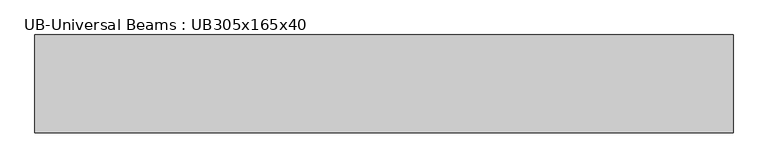
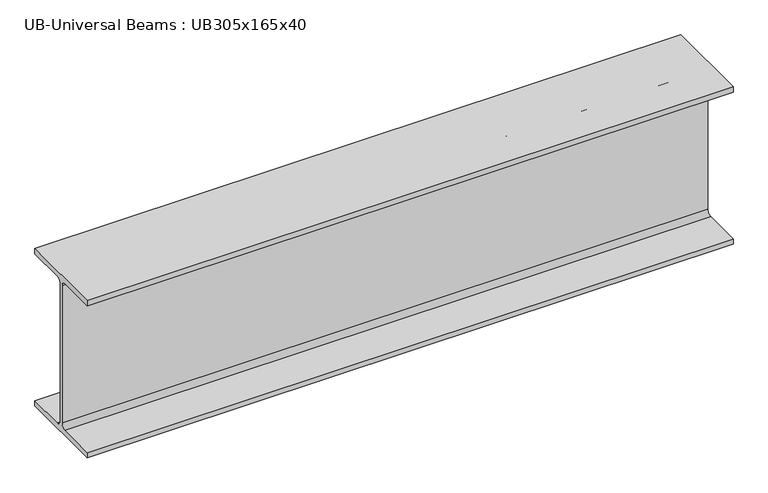
"""IFC4 building model written with IfcOpenShell, lengths in millimetres: beam geometry, UB-Universal Beams : UB305x165x40."""

from ifc_helpers import new_model, si_unit, point, frame, frame_2d, origin, place, context, project, spatial, polyline, circle_curve, trimmed, segment, composite_curve, outline, extrude, source, transform, mapped, element, save


def ub_universal_beams_ub305x165x40_a83b25bc(model_context):
    return source(origin(), model_context, "Body", "SweptSolid", [
        extrude(outline(composite_curve([segment(polyline([(82.5, -141.5), (82.5, -151.7), (-82.5, -151.7), (-82.5, -141.5), (-11.9, -141.5)]), True, "CONTINUOUS"), segment(trimmed(circle_curve(frame_2d((-11.9, -132.6)), 8.9), [point((-11.9, -141.5))], [point((-3.0, -132.6))], True, "CARTESIAN"), True, "CONTINUOUS"), segment(polyline([(-3.0, -132.6), (-3.0, 132.6)]), True, "CONTINUOUS"), segment(trimmed(circle_curve(frame_2d((-11.9, 132.6)), 8.9), [point((-3.0, 132.6))], [point((-11.9, 141.5))], True, "CARTESIAN"), True, "CONTINUOUS"), segment(polyline([(-11.9, 141.5), (-82.5, 141.5), (-82.5, 151.7), (82.5, 151.7), (82.5, 141.5), (11.9, 141.5)]), True, "CONTINUOUS"), segment(trimmed(circle_curve(frame_2d((11.9, 132.6)), 8.9), [point((11.9, 141.5))], [point((3.0, 132.6))], True, "CARTESIAN"), True, "CONTINUOUS"), segment(polyline([(3.0, 132.6), (3.0, -132.6)]), True, "CONTINUOUS"), segment(trimmed(circle_curve(frame_2d((11.9, -132.6)), 8.9), [point((3.0, -132.6))], [point((11.9, -141.5))], True, "CARTESIAN"), True, "CONTINUOUS"), segment(polyline([(11.9, -141.5), (82.5, -141.5)]), True, "CONTINUOUS")], self_intersect=False)), frame((-387.35, 0.0, 0.0), z_axis=(1.0, 0.0, 0.0), x_axis=(0.0, 1.0, 0.0)), (0.0, 0.0, 1.0), 1176.4),
    ])


if __name__ == "__main__":
    model = new_model("IFC4")
    model_context = context("Model", 3, world=origin())
    ifc_project = project(units=[si_unit("LENGTHUNIT", "METRE", prefix="MILLI")], contexts=[model_context])
    site = spatial("IfcSite", under=ifc_project)
    building = spatial("IfcBuilding", under=site)
    placement = place(None, origin())
    ub_universal_beams_ub305x165x40_shape = ub_universal_beams_ub305x165x40_a83b25bc(model_context)
    element("IfcBeam", 1, ObjectType="UB-Universal Beams : UB305x165x40", at=placement, inside=building, context=model_context, shape_type="MappedRepresentation", body=[
        mapped(ub_universal_beams_ub305x165x40_shape, transform((0.0, 0.0, 0.0), x_axis=(1.0, 0.0, 0.0), y_axis=(0.0, 1.0, 0.0), z_axis=(0.0, 0.0, 1.0))),
    ])
    save(model, "model.ifc")

# Revit data of these elements
# Type "UB-Universal Beams : UB305x165x40"
#   Section Name Key = "UB305X165X40"
#   Width = 16.5 cm
#   Web Thickness = 0.6 cm
#   Web Fillet = 0.89 cm
#   Warping Constant = 164000.0 cm⁶
#   Torsional Moment of Inertia = 14.70 cm⁴
#   Section Area = 51.3 cm²
#   Plastic Modulus weak axis = 142.0 cm³
#   Plastic Modulus strong axis = 623.0 cm³
#   Nominal Weight = 40.2999 kgf/m
#   Moment of Inertia weak axis = 764.00 cm⁴
#   Moment of Inertia strong axis = 8503.00 cm⁴
#   Height = 30.34 cm
#   Flange Thickness = 1.02 cm
#   Elastic Modulus weak axis = 92.6 cm³
#   Elastic Modulus strong axis = 560.0 cm³
#   Centroid Vertical = 15.17 cm
#   Centroid Horizontal = 8.25 cm
#   Bolt Spacing = 9.0 cm
#   Length [instance default] = 1500 mm
#   Structural Material [instance default] = Metal - Steel 43-275
#   Type Comments = ""
#   Assembly Code = ""
# Element 1 (IfcBeam, "UB-Universal Beams : UB305x165x40")
#   Materials on its faces: "Metal - Steel 43-275"
# Materials
#   "Metal - Steel 43-275": class "Metal", colour RGB 247 247 247, transparency 0, Cost = 0
